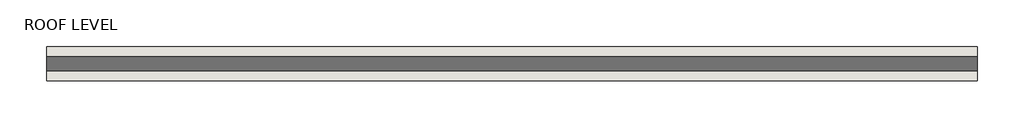
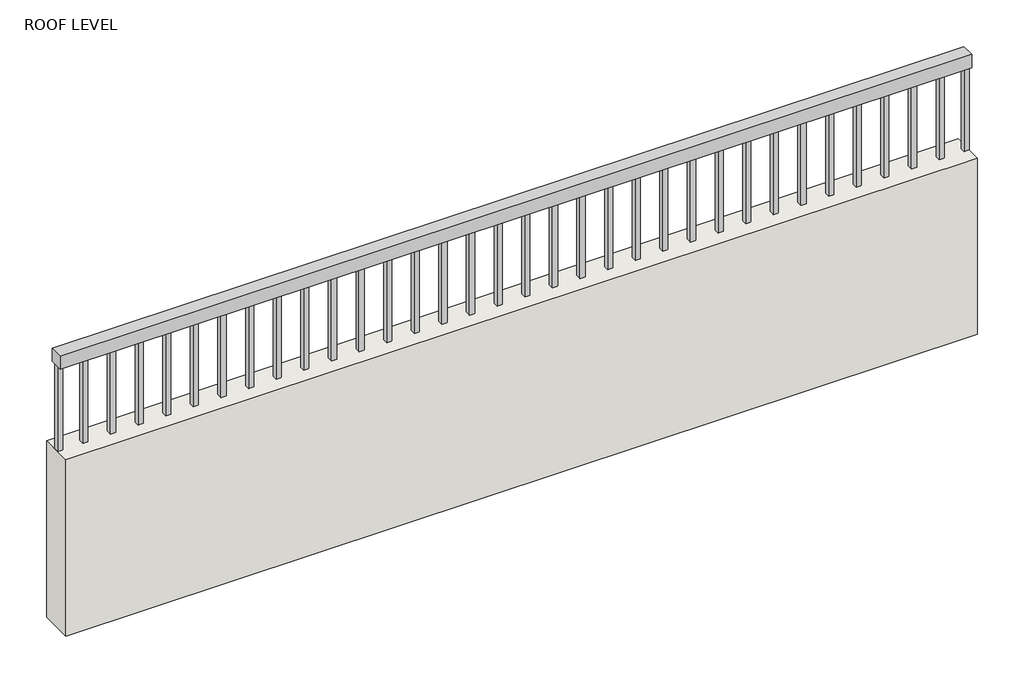
# One storey: 1 railing, 1 wall.
"""IFC4 building model written with IfcOpenShell, lengths in millimetres."""

from ifc_helpers import new_model, si_unit, frame, origin, place, context, project, spatial, polyline, outline, extrude, element, save

model = new_model("IFC4")

# Units and contexts
model_context = context("Model", 3, world=origin())
ifc_project = project(units=[si_unit("LENGTHUNIT", "METRE", prefix="MILLI")], contexts=[model_context])

# Site, building, storey
site = spatial("IfcSite", under=ifc_project)
building = spatial("IfcBuilding", under=site)
storey = spatial("IfcBuildingStorey", under=building, Name="ROOF LEVEL", Elevation=7924.8)

# Railing
placement = place(None, origin())
element("IfcRailing", 1, ObjectType="Handrail - Rectangular", at=placement, inside=storey, context=model_context, shape_type="SweptSolid", body=[
    extrude(outline(polyline([(-17501.168705, -11084.4152976), (-17501.168705, -11033.6152976), (-14148.368705, -11033.6152976), (-14148.368705, -11084.4152976), (-17501.168705, -11084.4152976)])), frame((0.0, 0.0, 9093.2), z_axis=(0.0, 0.0, 1.0), x_axis=(1.0, 0.0, 0.0)), (0.0, 0.0, 1.0), 50.8),
    extrude(outline(polyline([(-14259.493705, -11068.5402976), (-14259.493705, -11049.4902976), (-14240.443705, -11049.4902976), (-14240.443705, -11068.5402976), (-14259.493705, -11068.5402976)])), frame((0.0, 0.0, 8229.6), z_axis=(0.0, 0.0, 1.0), x_axis=(1.0, 0.0, 0.0)), (0.0, 0.0, 1.0), 863.6),
    extrude(outline(polyline([(-14361.093705, -11068.5402976), (-14361.093705, -11049.4902976), (-14342.043705, -11049.4902976), (-14342.043705, -11068.5402976), (-14361.093705, -11068.5402976)])), frame((0.0, 0.0, 8229.6), z_axis=(0.0, 0.0, 1.0), x_axis=(1.0, 0.0, 0.0)), (0.0, 0.0, 1.0), 863.6),
    extrude(outline(polyline([(-14462.693705, -11068.5402976), (-14462.693705, -11049.4902976), (-14443.643705, -11049.4902976), (-14443.643705, -11068.5402976), (-14462.693705, -11068.5402976)])), frame((0.0, 0.0, 8229.6), z_axis=(0.0, 0.0, 1.0), x_axis=(1.0, 0.0, 0.0)), (0.0, 0.0, 1.0), 863.6),
    extrude(outline(polyline([(-14564.293705, -11068.5402976), (-14564.293705, -11049.4902976), (-14545.243705, -11049.4902976), (-14545.243705, -11068.5402976), (-14564.293705, -11068.5402976)])), frame((0.0, 0.0, 8229.6), z_axis=(0.0, 0.0, 1.0), x_axis=(1.0, 0.0, 0.0)), (0.0, 0.0, 1.0), 863.6),
    extrude(outline(polyline([(-14665.893705, -11068.5402976), (-14665.893705, -11049.4902976), (-14646.843705, -11049.4902976), (-14646.843705, -11068.5402976), (-14665.893705, -11068.5402976)])), frame((0.0, 0.0, 8229.6), z_axis=(0.0, 0.0, 1.0), x_axis=(1.0, 0.0, 0.0)), (0.0, 0.0, 1.0), 863.6),
    extrude(outline(polyline([(-14767.493705, -11068.5402976), (-14767.493705, -11049.4902976), (-14748.443705, -11049.4902976), (-14748.443705, -11068.5402976), (-14767.493705, -11068.5402976)])), frame((0.0, 0.0, 8229.6), z_axis=(0.0, 0.0, 1.0), x_axis=(1.0, 0.0, 0.0)), (0.0, 0.0, 1.0), 863.6),
    extrude(outline(polyline([(-14869.093705, -11068.5402976), (-14869.093705, -11049.4902976), (-14850.043705, -11049.4902976), (-14850.043705, -11068.5402976), (-14869.093705, -11068.5402976)])), frame((0.0, 0.0, 8229.6), z_axis=(0.0, 0.0, 1.0), x_axis=(1.0, 0.0, 0.0)), (0.0, 0.0, 1.0), 863.6),
    extrude(outline(polyline([(-14970.693705, -11068.5402976), (-14970.693705, -11049.4902976), (-14951.643705, -11049.4902976), (-14951.643705, -11068.5402976), (-14970.693705, -11068.5402976)])), frame((0.0, 0.0, 8229.6), z_axis=(0.0, 0.0, 1.0), x_axis=(1.0, 0.0, 0.0)), (0.0, 0.0, 1.0), 863.6),
    extrude(outline(polyline([(-15072.293705, -11068.5402976), (-15072.293705, -11049.4902976), (-15053.243705, -11049.4902976), (-15053.243705, -11068.5402976), (-15072.293705, -11068.5402976)])), frame((0.0, 0.0, 8229.6), z_axis=(0.0, 0.0, 1.0), x_axis=(1.0, 0.0, 0.0)), (0.0, 0.0, 1.0), 863.6),
    extrude(outline(polyline([(-15173.893705, -11068.5402976), (-15173.893705, -11049.4902976), (-15154.843705, -11049.4902976), (-15154.843705, -11068.5402976), (-15173.893705, -11068.5402976)])), frame((0.0, 0.0, 8229.6), z_axis=(0.0, 0.0, 1.0), x_axis=(1.0, 0.0, 0.0)), (0.0, 0.0, 1.0), 863.6),
    extrude(outline(polyline([(-15275.493705, -11068.5402976), (-15275.493705, -11049.4902976), (-15256.443705, -11049.4902976), (-15256.443705, -11068.5402976), (-15275.493705, -11068.5402976)])), frame((0.0, 0.0, 8229.6), z_axis=(0.0, 0.0, 1.0), x_axis=(1.0, 0.0, 0.0)), (0.0, 0.0, 1.0), 863.6),
    extrude(outline(polyline([(-15377.093705, -11068.5402976), (-15377.093705, -11049.4902976), (-15358.043705, -11049.4902976), (-15358.043705, -11068.5402976), (-15377.093705, -11068.5402976)])), frame((0.0, 0.0, 8229.6), z_axis=(0.0, 0.0, 1.0), x_axis=(1.0, 0.0, 0.0)), (0.0, 0.0, 1.0), 863.6),
    extrude(outline(polyline([(-15478.693705, -11068.5402976), (-15478.693705, -11049.4902976), (-15459.643705, -11049.4902976), (-15459.643705, -11068.5402976), (-15478.693705, -11068.5402976)])), frame((0.0, 0.0, 8229.6), z_axis=(0.0, 0.0, 1.0), x_axis=(1.0, 0.0, 0.0)), (0.0, 0.0, 1.0), 863.6),
    extrude(outline(polyline([(-15580.293705, -11068.5402976), (-15580.293705, -11049.4902976), (-15561.243705, -11049.4902976), (-15561.243705, -11068.5402976), (-15580.293705, -11068.5402976)])), frame((0.0, 0.0, 8229.6), z_axis=(0.0, 0.0, 1.0), x_axis=(1.0, 0.0, 0.0)), (0.0, 0.0, 1.0), 863.6),
    extrude(outline(polyline([(-15681.893705, -11068.5402976), (-15681.893705, -11049.4902976), (-15662.843705, -11049.4902976), (-15662.843705, -11068.5402976), (-15681.893705, -11068.5402976)])), frame((0.0, 0.0, 8229.6), z_axis=(0.0, 0.0, 1.0), x_axis=(1.0, 0.0, 0.0)), (0.0, 0.0, 1.0), 863.6),
    extrude(outline(polyline([(-15783.493705, -11068.5402976), (-15783.493705, -11049.4902976), (-15764.443705, -11049.4902976), (-15764.443705, -11068.5402976), (-15783.493705, -11068.5402976)])), frame((0.0, 0.0, 8229.6), z_axis=(0.0, 0.0, 1.0), x_axis=(1.0, 0.0, 0.0)), (0.0, 0.0, 1.0), 863.6),
    extrude(outline(polyline([(-15885.093705, -11068.5402976), (-15885.093705, -11049.4902976), (-15866.043705, -11049.4902976), (-15866.043705, -11068.5402976), (-15885.093705, -11068.5402976)])), frame((0.0, 0.0, 8229.6), z_axis=(0.0, 0.0, 1.0), x_axis=(1.0, 0.0, 0.0)), (0.0, 0.0, 1.0), 863.6),
    extrude(outline(polyline([(-15986.693705, -11068.5402976), (-15986.693705, -11049.4902976), (-15967.643705, -11049.4902976), (-15967.643705, -11068.5402976), (-15986.693705, -11068.5402976)])), frame((0.0, 0.0, 8229.6), z_axis=(0.0, 0.0, 1.0), x_axis=(1.0, 0.0, 0.0)), (0.0, 0.0, 1.0), 863.6),
    extrude(outline(polyline([(-16088.293705, -11068.5402976), (-16088.293705, -11049.4902976), (-16069.243705, -11049.4902976), (-16069.243705, -11068.5402976), (-16088.293705, -11068.5402976)])), frame((0.0, 0.0, 8229.6), z_axis=(0.0, 0.0, 1.0), x_axis=(1.0, 0.0, 0.0)), (0.0, 0.0, 1.0), 863.6),
    extrude(outline(polyline([(-16189.893705, -11068.5402976), (-16189.893705, -11049.4902976), (-16170.843705, -11049.4902976), (-16170.843705, -11068.5402976), (-16189.893705, -11068.5402976)])), frame((0.0, 0.0, 8229.6), z_axis=(0.0, 0.0, 1.0), x_axis=(1.0, 0.0, 0.0)), (0.0, 0.0, 1.0), 863.6),
    extrude(outline(polyline([(-16291.493705, -11068.5402976), (-16291.493705, -11049.4902976), (-16272.443705, -11049.4902976), (-16272.443705, -11068.5402976), (-16291.493705, -11068.5402976)])), frame((0.0, 0.0, 8229.6), z_axis=(0.0, 0.0, 1.0), x_axis=(1.0, 0.0, 0.0)), (0.0, 0.0, 1.0), 863.6),
    extrude(outline(polyline([(-16393.093705, -11068.5402976), (-16393.093705, -11049.4902976), (-16374.043705, -11049.4902976), (-16374.043705, -11068.5402976), (-16393.093705, -11068.5402976)])), frame((0.0, 0.0, 8229.6), z_axis=(0.0, 0.0, 1.0), x_axis=(1.0, 0.0, 0.0)), (0.0, 0.0, 1.0), 863.6),
    extrude(outline(polyline([(-16494.693705, -11068.5402976), (-16494.693705, -11049.4902976), (-16475.643705, -11049.4902976), (-16475.643705, -11068.5402976), (-16494.693705, -11068.5402976)])), frame((0.0, 0.0, 8229.6), z_axis=(0.0, 0.0, 1.0), x_axis=(1.0, 0.0, 0.0)), (0.0, 0.0, 1.0), 863.6),
    extrude(outline(polyline([(-16596.293705, -11068.5402976), (-16596.293705, -11049.4902976), (-16577.243705, -11049.4902976), (-16577.243705, -11068.5402976), (-16596.293705, -11068.5402976)])), frame((0.0, 0.0, 8229.6), z_axis=(0.0, 0.0, 1.0), x_axis=(1.0, 0.0, 0.0)), (0.0, 0.0, 1.0), 863.6),
    extrude(outline(polyline([(-16697.893705, -11068.5402976), (-16697.893705, -11049.4902976), (-16678.843705, -11049.4902976), (-16678.843705, -11068.5402976), (-16697.893705, -11068.5402976)])), frame((0.0, 0.0, 8229.6), z_axis=(0.0, 0.0, 1.0), x_axis=(1.0, 0.0, 0.0)), (0.0, 0.0, 1.0), 863.6),
    extrude(outline(polyline([(-16799.493705, -11068.5402976), (-16799.493705, -11049.4902976), (-16780.443705, -11049.4902976), (-16780.443705, -11068.5402976), (-16799.493705, -11068.5402976)])), frame((0.0, 0.0, 8229.6), z_axis=(0.0, 0.0, 1.0), x_axis=(1.0, 0.0, 0.0)), (0.0, 0.0, 1.0), 863.6),
    extrude(outline(polyline([(-16901.093705, -11068.5402976), (-16901.093705, -11049.4902976), (-16882.043705, -11049.4902976), (-16882.043705, -11068.5402976), (-16901.093705, -11068.5402976)])), frame((0.0, 0.0, 8229.6), z_axis=(0.0, 0.0, 1.0), x_axis=(1.0, 0.0, 0.0)), (0.0, 0.0, 1.0), 863.6),
    extrude(outline(polyline([(-17002.693705, -11068.5402976), (-17002.693705, -11049.4902976), (-16983.643705, -11049.4902976), (-16983.643705, -11068.5402976), (-17002.693705, -11068.5402976)])), frame((0.0, 0.0, 8229.6), z_axis=(0.0, 0.0, 1.0), x_axis=(1.0, 0.0, 0.0)), (0.0, 0.0, 1.0), 863.6),
    extrude(outline(polyline([(-17104.293705, -11068.5402976), (-17104.293705, -11049.4902976), (-17085.243705, -11049.4902976), (-17085.243705, -11068.5402976), (-17104.293705, -11068.5402976)])), frame((0.0, 0.0, 8229.6), z_axis=(0.0, 0.0, 1.0), x_axis=(1.0, 0.0, 0.0)), (0.0, 0.0, 1.0), 863.6),
    extrude(outline(polyline([(-17205.893705, -11068.5402976), (-17205.893705, -11049.4902976), (-17186.843705, -11049.4902976), (-17186.843705, -11068.5402976), (-17205.893705, -11068.5402976)])), frame((0.0, 0.0, 8229.6), z_axis=(0.0, 0.0, 1.0), x_axis=(1.0, 0.0, 0.0)), (0.0, 0.0, 1.0), 863.6),
    extrude(outline(polyline([(-17307.493705, -11068.5402976), (-17307.493705, -11049.4902976), (-17288.443705, -11049.4902976), (-17288.443705, -11068.5402976), (-17307.493705, -11068.5402976)])), frame((0.0, 0.0, 8229.6), z_axis=(0.0, 0.0, 1.0), x_axis=(1.0, 0.0, 0.0)), (0.0, 0.0, 1.0), 863.6),
    extrude(outline(polyline([(-17409.093705, -11068.5402976), (-17409.093705, -11049.4902976), (-17390.043705, -11049.4902976), (-17390.043705, -11068.5402976), (-17409.093705, -11068.5402976)])), frame((0.0, 0.0, 8229.6), z_axis=(0.0, 0.0, 1.0), x_axis=(1.0, 0.0, 0.0)), (0.0, 0.0, 1.0), 863.6),
    extrude(outline(polyline([(-14167.418705, -11068.5402976), (-14167.418705, -11049.4902976), (-14148.368705, -11049.4902976), (-14148.368705, -11068.5402976), (-14167.418705, -11068.5402976)])), frame((0.0, 0.0, 8229.6), z_axis=(0.0, 0.0, 1.0), x_axis=(1.0, 0.0, 0.0)), (0.0, 0.0, 1.0), 863.6),
    extrude(outline(polyline([(-17501.168705, -11068.5402976), (-17501.168705, -11049.4902976), (-17482.118705, -11049.4902976), (-17482.118705, -11068.5402976), (-17501.168705, -11068.5402976)])), frame((0.0, 0.0, 8229.6), z_axis=(0.0, 0.0, 1.0), x_axis=(1.0, 0.0, 0.0)), (0.0, 0.0, 1.0), 863.6),
])

# Wall
element("IfcWall", 2, ObjectType="Interior - 4 7/8\" Partition (1-hr) 2", at=placement, inside=storey, context=model_context, shape_type="SweptSolid", body=[
    extrude(outline(polyline([(-14148.368705, -11120.9277976), (-17501.168705, -11120.9277976), (-17501.168705, -10997.1027976), (-14148.368705, -10997.1027976), (-14148.368705, -11120.9277976)])), frame((0.0, 0.0, 8077.2), z_axis=(0.0, 0.0, 1.0), x_axis=(1.0, 0.0, 0.0)), (0.0, 0.0, 1.0), 685.8),
])

save(model, "model.ifc")

# Revit data of these elements
# Type "Handrail - Rectangular"
#   Assembly Code = "C2010400"
#   built-in parameter 1008612 = 0.0416667 (stored number, unit not read)
#   built-in parameter 1008611 = 0.0416667 (stored number, unit not read)
#   built-in parameter 1008609 = 0.333333 (stored number, unit not read)
#   built-in parameter 1008604 = 0.166667 (stored number, unit not read)
#   built-in parameter 1008603 = 0.166667 (stored number, unit not read)
#   Railing Height = 3' - 0"
#   built-in parameter 1008630 = 2
#   built-in parameter 1008610 = 2
#   built-in parameter 1008618 = Baluster - Square : 3/4"
# Type "Interior - 4 7/8\" Partition (1-hr) 2"
#   Assembly Code = "C1010145"
# Element 1 (IfcRailing, "Handrail - Rectangular")
#   built-in parameter 1008621 = 1 (stored number, unit not read)
#   Phase Created = New Construction
# Element 2 (IfcWall, "Interior - 4 7/8\" Partition (1-hr) 2")
#   built-in parameter 1001111 = 0' - 6"
#   Top Offset = 0' - 0"
#   Base Offset = 0' - 6"
#   Unconnected Height = 2' - 3"
#   wall height = 2' - 3"
#   Phase Created = New Construction
#   Base Constraint = ROOF LEVEL
#   Materials on its faces: "Default Wall"
# Materials
#   "Default Wall": colour RGB 128 128 128, transparency 0, Cost = 0
